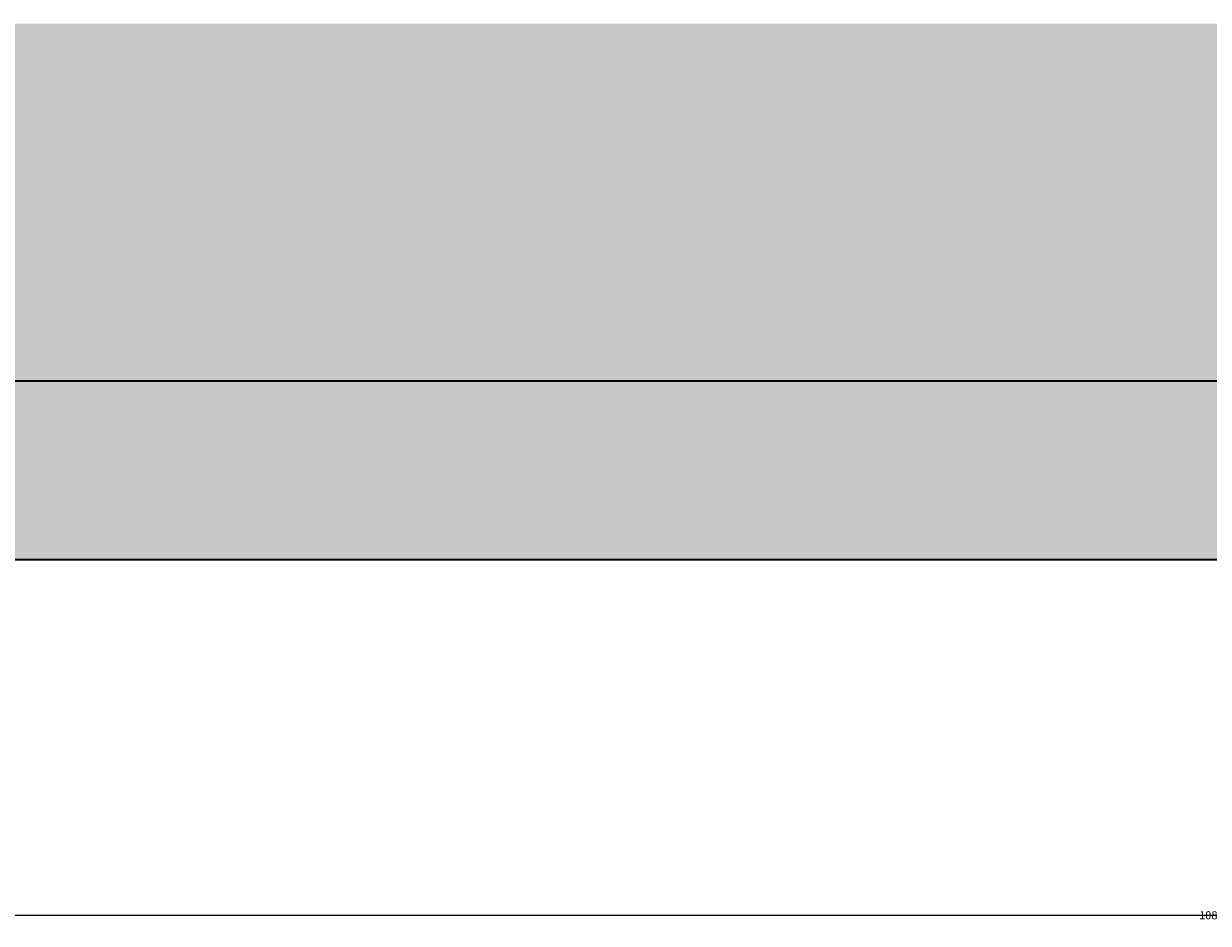
# Model space of a CAD drawing. Units: inches. Extents: x 4508 to 4723, y 847 to 1020.
# Tile 4 of 32: x 4577 to 4604, y 867 to 887. Entities that reach past the tile are written whole.
import ezdxf

# ---------------------------------------------------------------- set-up
doc = ezdxf.new("R2010")
doc.units = ezdxf.units.IN
for name, color, linetype, lineweight in [('A-ANNO-DIMS', 2, 'Continuous', 18), ('A-WALL', 7, 'Continuous', 35), ('A-WALL-PATT', 254, 'Continuous', 13)]:
    doc.layers.add(name, color=color, linetype=linetype, lineweight=lineweight)
doc.styles.get("Standard").update_dxf_attribs({"font": 'arial.ttf'})
doc.dimstyles.get("Standard").update_dxf_attribs({"dimtxt": 0.18, "dimasz": 0.18, "dimexe": 0.18, "dimexo": 0.0625, "dimgap": 0.09, "dimtad": 0, "dimtih": 1, "dimtoh": 1, "dimdec": 4, "dimzin": 0, "dimdsep": 46, "dimtxsty": 'Standard', "dimcen": 0.09, "dimadec": 0, "dimazin": 0, "dimtfac": 1, "dimtdec": 4, "dimtofl": 0, "dimtmove": 0, "dimatfit": 3, "dimfxl": 1, "dimtolj": 1, "dimtzin": 0, "dimarcsym": 0})

# ---------------------------------------------------------------- blocks, each defined once
blk = doc.blocks.new('*D2')
at = {"layer": 'A-ANNO-DIMS', "color": 0, "lineweight": -2, "transparency": 16777216}
for p, q in [((4540.994, 874.684), (4540.994, 866.617)), ((4693.994, 874.684), (4693.994, 866.617)), ((4541.174, 866.797), (4617.213, 866.797)), ((4693.814, 866.797), (4617.774, 866.797))]:
    blk.add_line(p, q, dxfattribs=at)
at = {"layer": 'A-ANNO-DIMS', "color": 0, "lineweight": 9, "transparency": 16777216}
for points in [[(4541.174, 866.827), (4541.174, 866.767), (4540.994, 866.797)], [(4693.814, 866.827), (4693.814, 866.767), (4693.994, 866.797)]]:
    blk.add_solid(points, dxfattribs=at)
at = {"layer": 'Defpoints', "color": 0, "lineweight": 9, "transparency": 16777216}
for p in [(4540.994, 874.747), (4693.994, 874.747), (4693.994, 866.797)]:
    blk.add_point(p, dxfattribs=at)
at = {"layer": 'A-ANNO-DIMS', "color": 0, "transparency": 16777216, "insert": (4617.494, 866.797), "char_height": 0.18, "attachment_point": 5}
blk.add_mtext('\\A1;153', dxfattribs=at)
blk = doc.blocks.new('*D24')
at = {"layer": 'A-ANNO-DIMS', "color": 0, "lineweight": -2, "transparency": 16777216}
for p, q in [((4549.994, 886.684), (4549.994, 866.617)), ((4657.994, 886.684), (4657.994, 866.617)), ((4550.174, 866.797), (4603.713, 866.797)), ((4657.814, 866.797), (4604.274, 866.797))]:
    blk.add_line(p, q, dxfattribs=at)
at = {"layer": 'A-ANNO-DIMS', "color": 0, "lineweight": 9, "transparency": 16777216}
for points in [[(4550.174, 866.827), (4550.174, 866.767), (4549.994, 866.797)], [(4657.814, 866.827), (4657.814, 866.767), (4657.994, 866.797)]]:
    blk.add_solid(points, dxfattribs=at)
at = {"layer": 'Defpoints', "color": 0, "lineweight": 9, "transparency": 16777216}
for p in [(4549.994, 886.747), (4657.994, 886.747), (4657.994, 866.797)]:
    blk.add_point(p, dxfattribs=at)
at = {"layer": 'A-ANNO-DIMS', "color": 0, "transparency": 16777216, "insert": (4603.994, 866.797), "char_height": 0.18, "attachment_point": 5}
blk.add_mtext('\\A1;108', dxfattribs=at)

msp = doc.modelspace()

# ---------------------------------------------------------------- hatches: boundary and pattern name
at = {"layer": 'A-WALL-PATT', "transparency": 33554508}
h = msp.add_hatch(color=256, dxfattribs=at)
h.dxf.hatch_style = 1
h.paths.add_polyline_path([(4661.6706, 954.043, -0.3739004), (4658.5765, 957.6021, -1), (4665.7646, 957.6021, -0.3739004), (4662.6706, 954.043), (4662.6706, 944.4021, -0.2114781), (4670.3062, 945.0869), (4670.3062, 968.0592, -0.4632086), (4663.3246, 973.9783, -0.4632086), (4670.3062, 979.8975), (4670.3062, 994.7469), (4588.9938, 994.7469), (4588.9938, 904.7469), (4657.9938, 904.7469), (4657.9938, 886.7469), (4549.9938, 886.7469), (4549.9938, 878.7469), (4693.9938, 878.7469), (4693.9938, 994.7469), (4671.8062, 994.7469), (4671.8062, 979.4411, -0.2941682), (4675.3246, 973.9783, -0.2941682), (4671.8062, 968.5156), (4671.8062, 944.4278, -0.2741114), (4676.7298, 936.1217, -0.2741114), (4671.8062, 927.8155), (4671.8062, 907.6998, -0.3779645), (4677.0562, 901.7469, -0.3779645), (4671.8062, 895.7939), (4671.8062, 883.7469), (4670.3062, 883.7469), (4670.3062, 895.7939, -0.3779645), (4665.0562, 901.7469, -0.3779645), (4670.3062, 907.6998), (4670.3062, 927.1564, -0.2114781), (4662.6706, 927.8412), (4662.6706, 918.2003, -0.3739004), (4665.7646, 914.6412, -1), (4658.5765, 914.6412, -0.3739004), (4661.6706, 918.2003), (4661.6706, 928.4807, -0.2391825), (4657.7936, 936.1217, -0.2391825), (4661.6706, 943.7626)])
at = {"layer": 'A-WALL-PATT', "transparency": 33554556}
h = msp.add_hatch(color=256, dxfattribs=at)
h.dxf.hatch_style = 1
h.paths.add_polyline_path([(4689.9938, 878.7469), (4549.9938, 878.7469), (4549.9938, 874.7469), (4689.9938, 874.7469)])

# ---------------------------------------------------------------- linework, layer by layer
at = {"layer": 'A-WALL'}
for p, q in [((4693.9938, 878.7469), (4549.9938, 878.7469)), ((4693.9938, 874.7469), (4549.9938, 874.7469))]:
    msp.add_line(p, q, dxfattribs=at)

# ---------------------------------------------------------------- dimensions: what is measured, and where the dimension line sits
at = {"layer": 'A-ANNO-DIMS'}
for base, p1, p2, picture, middle in [((4657.9938, 866.7969), (4549.9938, 886.7469), (4657.9938, 886.7469), '*D24', (4603.9938, 866.7969)), ((4693.9938, 866.7969), (4540.9938, 874.7469), (4693.9938, 874.7469), '*D2', (4617.4938, 866.7969))]:
    dim = msp.add_linear_dim(base=base, p1=p1, p2=p2, dimstyle='Standard', override={"dimdec": 0, "dimlfac": 1, "dimrnd": 0, "dimzin": 0, "dimdsep": 46, "dimlunit": 2}, dxfattribs=at)
    dim.commit()
    dim.dimension.update_dxf_attribs({"geometry": picture, "text_midpoint": middle})

doc.saveas('drawing.dxf')
